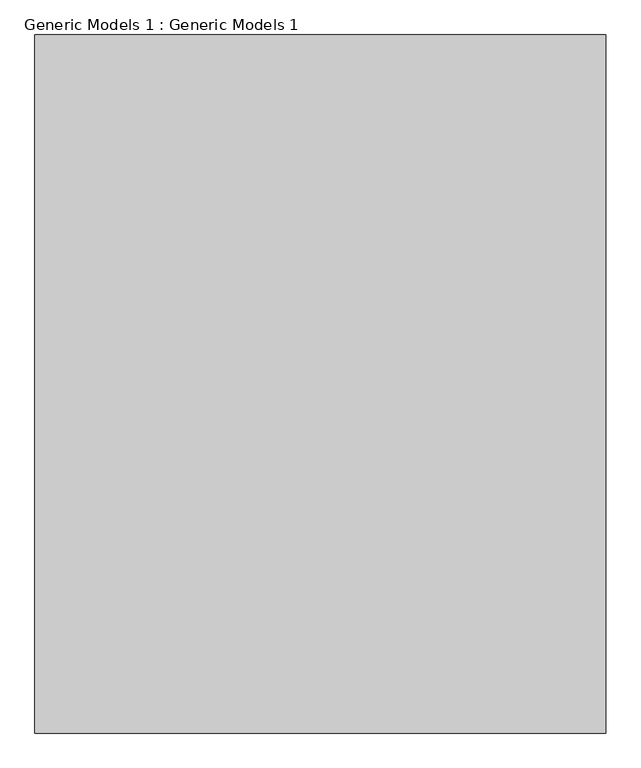
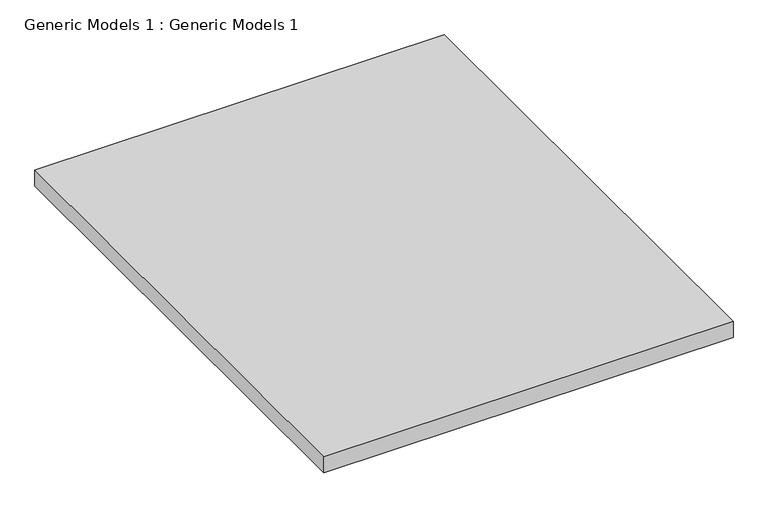
"""IFC4 building model written with IfcOpenShell, lengths in millimetres: proxy geometry, Generic Models 1 : Generic Models 1."""

from ifc_helpers import new_model, si_unit, frame, origin, place, context, project, spatial, polyline, outline, extrude, source, transform, mapped, element, save


def generic_models_1_generic_models_1_4ef364dd(model_context):
    return source(origin(), model_context, "Body", "SweptSolid", [
        extrude(outline(polyline([(-17947.3642027, -7514.2678797), (-17947.3642027, -4479.7618509), (-15465.7261518, -4479.7618509), (-15465.7261518, -7514.2678797), (-17947.3642027, -7514.2678797)])), frame((0.0, 0.0, -152.4), z_axis=(0.0, 0.0, 1.0), x_axis=(1.0, 0.0, 0.0)), (0.0, 0.0, 1.0), 101.6),
    ])


if __name__ == "__main__":
    model = new_model("IFC4")
    model_context = context("Model", 3, world=origin())
    ifc_project = project(units=[si_unit("LENGTHUNIT", "METRE", prefix="MILLI")], contexts=[model_context])
    site = spatial("IfcSite", under=ifc_project)
    building = spatial("IfcBuilding", under=site)
    placement = place(None, origin())
    generic_models_1_generic_models_1_shape = generic_models_1_generic_models_1_4ef364dd(model_context)
    element("IfcBuildingElementProxy", 1, Name="Generic Models 1 : Generic Models 1", ObjectType="Generic Models 1 : Generic Models 1", at=placement, inside=building, context=model_context, shape_type="MappedRepresentation", body=[
        mapped(generic_models_1_generic_models_1_shape, transform((0.0, 0.0, 0.0), x_axis=(1.0, 0.0, 0.0), y_axis=(0.0, 1.0, 0.0), z_axis=(0.0, 0.0, 1.0))),
    ])
    save(model, "model.ifc")

# Revit data of these elements
# Element 1 (IfcBuildingElementProxy, "Generic Models 1 : Generic Models 1")
#   Materials on its faces: "PARKING"
# Materials
#   "PARKING": class "Generic", colour RGB 120 120 120, transparency 0, Cost = 0
